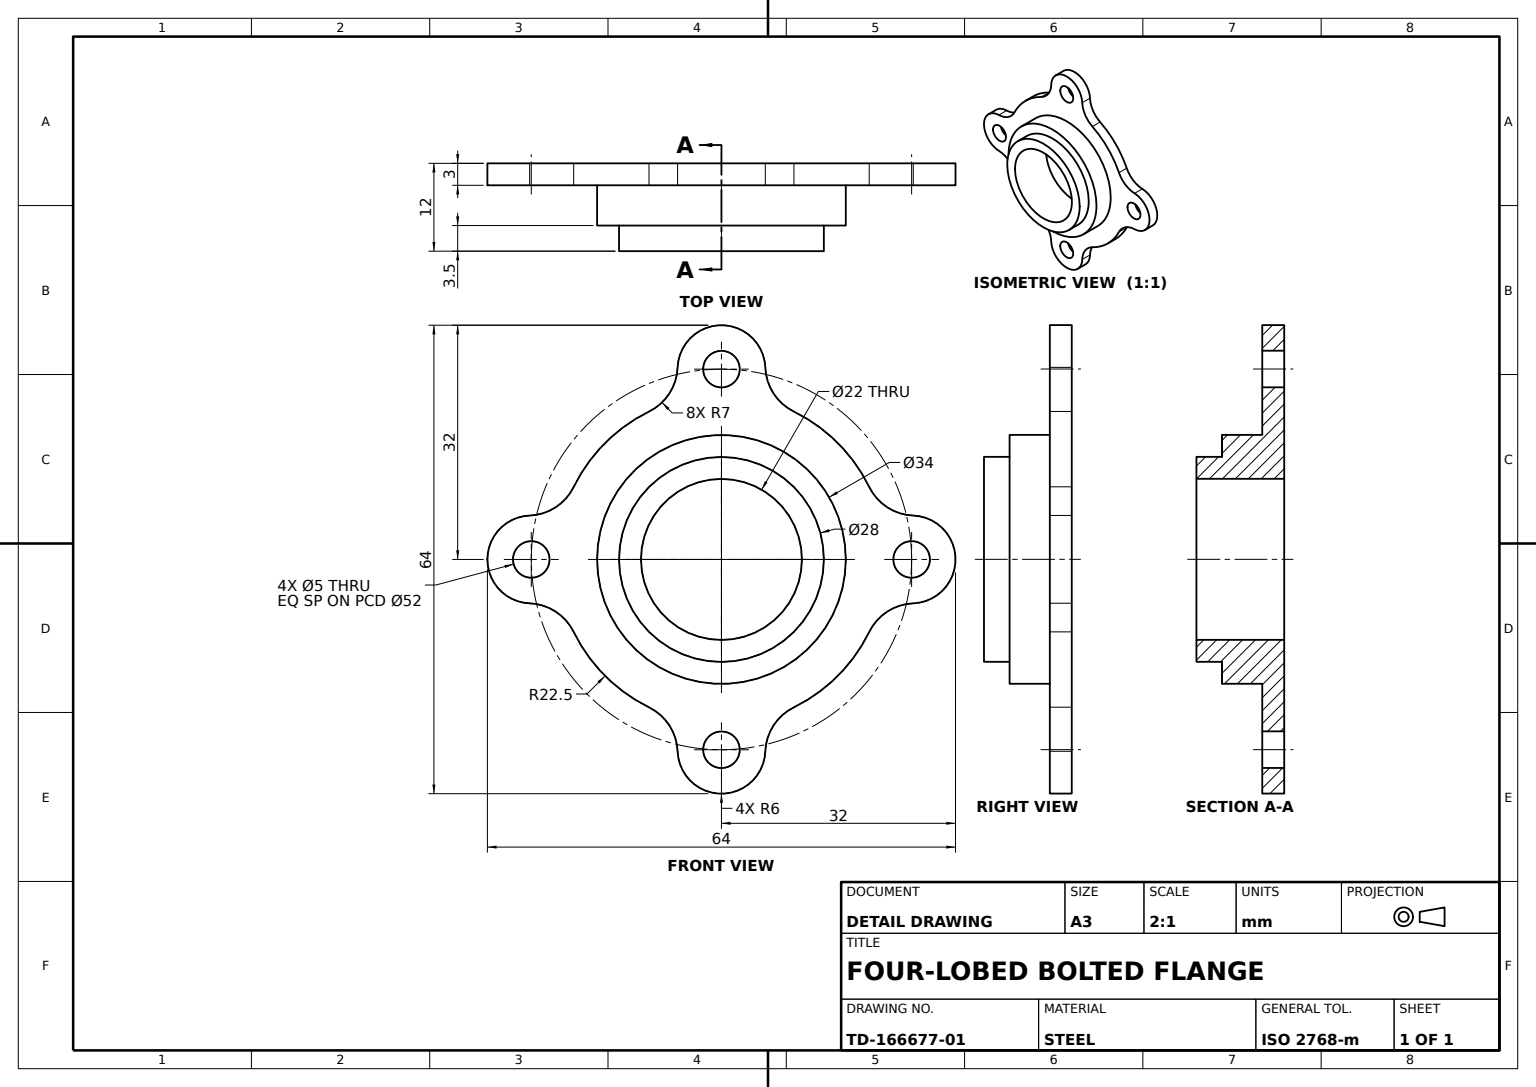
SolidWorks part; units mm, degrees
material "Plain Carbon Steel"
ref_plane "Front Plane" through (0, 0, 0) normal (0, 0, 1) x (1, 0, 0)
ref_plane "Top Plane" through (0, 0, 0) normal (0, 1, 0) x (1, 0, 0)
ref_plane "Right Plane" through (0, 0, 0) normal (1, 0, 0) x (0, 0, -1)
sketch "Flange Profile Sketch" plane through (0, 0, 0) normal (0, 0, 1) x (1, 0, 0)
  arc A0 (9.9083, -20.2009) -> (20.2009, -9.9083) centre (0, 0) ccw
  arc A2 (26.2241, -5.9958) -> (26.2241, 5.9958) centre (26, 0) ccw
  arc A3 (5.9958, 26.2241) -> (-5.9958, 26.2241) centre (0, 26) ccw
  arc A4 (-26.2241, 5.9958) -> (-26.2241, -5.9958) centre (-26, 0) ccw
  arc A5 (-5.9958, -26.2241) -> (5.9958, -26.2241) centre (0, -26) ccw
  arc A6 (20.2009, 9.9083) -> (9.9083, 20.2009) centre (0, 0) ccw
  arc A7 (-9.9083, 20.2009) -> (-20.2009, 9.9083) centre (0, 0) ccw
  arc A8 (-20.2009, -9.9083) -> (-9.9083, -20.2009) centre (0, 0) ccw
  arc A9 (9.9083, 20.2009) -> (5.9958, 26.2241) centre (12.9909, 26.4856) cw
  arc A10 (-5.9958, -26.2241) -> (-9.9083, -20.2009) centre (-12.9909, -26.4856) ccw
  arc A11 (-20.2009, -9.9083) -> (-26.2241, -5.9958) centre (-26.4856, -12.9909) ccw
  arc A12 (-20.2009, 9.9083) -> (-26.2241, 5.9958) centre (-26.4856, 12.9909) cw
  arc A13 (-5.9958, 26.2241) -> (-9.9083, 20.2009) centre (-12.9909, 26.4856) cw
  arc A14 (26.2241, 5.9958) -> (20.2009, 9.9083) centre (26.4856, 12.9909) cw
  arc A15 (26.2241, -5.9958) -> (20.2009, -9.9083) centre (26.4856, -12.9909) ccw
  arc A16 (9.9083, -20.2009) -> (5.9958, -26.2241) centre (12.9909, -26.4856) ccw
  point P15 (4.5105, 22.0433)
  point P21 (-22.0433, -4.5105)
  point P24 (-22.0433, 4.5105)
  point P27 (-4.5105, 22.0433)
  point P30 (22.0433, 4.5105)
  dimension "D1" = 22.5
  dimension "D2" = 7
  dimension "D7" = 6
  dimension "D8" = 6
  dimension "D9" = 6
  dimension "D10" = 6
  dimension "D3" = 7
  dimension "D4" = 7
  dimension "D5" = 16.3158
  dimension "D6" = 3.9125
  dimension "D11" = 3.9125
  dimension "D12" = 6.0232
extrude "Lug Flange" add sketch "Flange Profile Sketch" along normal blind 3
sketch "Hub Sketch" plane through (0, 0, 3) normal (0, 0, 1) x (1, 0, 0)
  circle A0 centre (0, 0) radius 17
  dimension "D1" = 17
extrude "Hub Boss" add sketch "Hub Sketch" along normal blind 5.5
sketch "Spigot Sketch" plane through (0, 0, 8.5) normal (0, 0, 1) x (1, 0, 0)
  circle A0 centre (0, 0) radius 14
  dimension "D1" = 14
extrude "Locating Spigot" add sketch "Spigot Sketch" along normal blind 3.5
sketch "Bearing Bore Sketch" plane through (0, 0, 12) normal (0, 0, 1) x (1, 0, 0)
  circle A0 centre (0, 0) radius 11
  dimension "D1" = 11
extrude "Bearing Bore" cut sketch "Bearing Bore Sketch" against normal blind 15
sketch "Lug Holes Sketch" plane through (0, 0, 3) normal (0, 0, 1) x (1, 0, 0)
  circle A0 centre (-26, 0) radius 2.5
  circle A1 centre (0, 26) radius 2.5
  circle A2 centre (26, 0) radius 2.5
  circle A3 centre (0, -26) radius 2.5
  dimension "D1" = 2.5
  dimension "D2" = 2.5
  dimension "D3" = 2.5
  dimension "D4" = 2.5
extrude "Lug Mounting Holes 4x" cut sketch "Lug Holes Sketch" against normal blind 15
